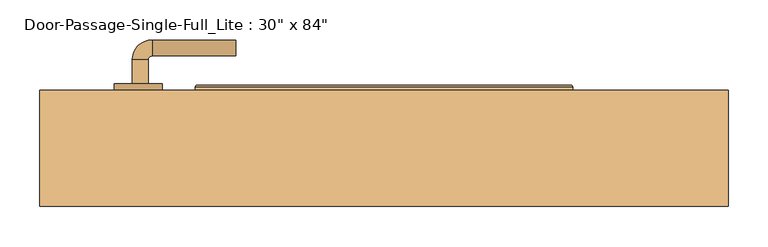
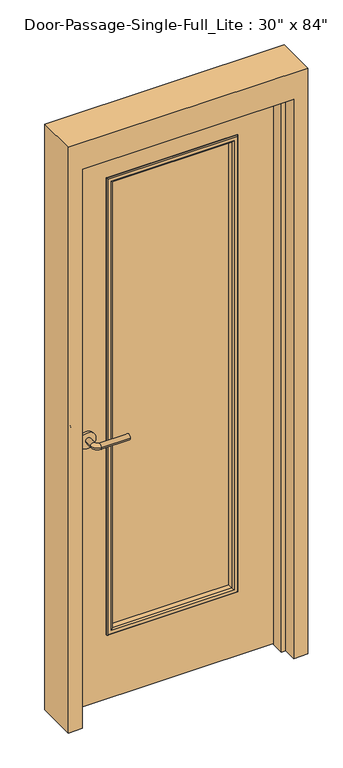
"""IFC4 building model written with IfcOpenShell, lengths in millimetres: door geometry."""

from ifc_helpers import new_model, si_unit, point, frame, frame_2d, origin, place, context, project, spatial, polyline, circle_curve, ellipse_curve, trimmed, segment, composite_curve, outline, extrude, faceted_brep, source, transform, mapped, element, save
from ifc_brep_helpers import plane_surface, cylinder_surface, revolved_surface, advanced_brep


def door_5761e9ac(model_context):
    return source(origin(), model_context, "Body", "SolidModel", [
        advanced_brep(
        [(-315.990625, 42.8, 1016.0), (-295.990625, 42.8, 1016.0), (-295.990625, 12.8, 1016.0), (-315.990625, 12.8, 1016.0), (-290.990625, 7.8, 1016.0), (-290.990625, -12.2, 1016.0), (-185.990625, -12.2, 1016.0), (-185.990625, 7.8, 1016.0)],
        [
            (0, 1, circle_curve(frame((-305.990625, 42.8, 1016.0), z_axis=(0.0, 1.0, 0.0), x_axis=(1.0, 0.0, 0.0)), 10.0)),
            (1, 0, circle_curve(frame((-305.990625, 42.8, 1016.0), z_axis=(0.0, 1.0, 0.0), x_axis=(1.0, 0.0, 0.0)), 10.0)),
            (1, 2),
            (2, 3, circle_curve(frame((-305.990625, 12.8, 1016.0), z_axis=(0.0, 1.0, 0.0), x_axis=(1.0, 0.0, 0.0)), 10.0)),
            (3, 0),
            (3, 2, circle_curve(frame((-305.990625, 12.8, 1016.0), z_axis=(0.0, 1.0, 0.0), x_axis=(1.0, 0.0, 0.0)), 10.0)),
            (4, 5, circle_curve(frame((-290.990625, -2.2, 1016.0), z_axis=(-1.0, 0.0, 0.0), x_axis=(0.0, 1.0, 0.0)), 10.0)),
            (5, 3, circle_curve(frame((-290.990625, 12.8, 1016.0), z_axis=(0.0, 0.0, -1.0), x_axis=(-1.0, 0.0, 0.0)), 25.0)),
            (2, 4, circle_curve(frame((-290.990625, 12.8, 1016.0), z_axis=(0.0, 0.0, 1.0), x_axis=(-1.0, 0.0, 0.0)), 5.0)),
            (5, 4, circle_curve(frame((-290.990625, -2.2, 1016.0), z_axis=(-1.0, 0.0, 0.0), x_axis=(0.0, 1.0, 0.0)), 10.0)),
            (6, 7, circle_curve(frame((-185.990625, -2.2, 1016.0), z_axis=(1.0, 0.0, 0.0), x_axis=(0.0, 1.0, 0.0)), 10.0)),
            (7, 6, circle_curve(frame((-185.990625, -2.2, 1016.0), z_axis=(1.0, 0.0, 0.0), x_axis=(0.0, 1.0, 0.0)), 10.0)),
            (4, 7),
            (6, 5),
        ],
        [
            plane_surface(frame((-305.990625, 42.8, 1016.0), z_axis=(0.0, 1.0, 0.0), x_axis=(0.0, 0.0, 1.0))),
            cylinder_surface(frame((-305.990625, 42.8, 1016.0), z_axis=(0.0, 1.0, 0.0), x_axis=(1.0, 0.0, 0.0)), 10.0),
            revolved_surface(trimmed(ellipse_curve(frame((-305.990625, 12.8, 1016.0), z_axis=(0.0, -1.0, 0.0), x_axis=(1.0, 0.0, 0.0)), 10.0, 10.0), [point((-315.990625, 12.8, 1016.0))], [point((-295.990625, 12.8, 1016.0))], True, "CARTESIAN"), (-290.990625, 12.8, 1016.0), (0.0, 0.0, -1.0)),
            revolved_surface(trimmed(ellipse_curve(frame((-305.990625, 12.8, 1016.0), z_axis=(0.0, -1.0, 0.0), x_axis=(1.0, 0.0, 0.0)), 10.0, 10.0), [point((-295.990625, 12.8, 1016.0))], [point((-315.990625, 12.8, 1016.0))], True, "CARTESIAN"), (-290.990625, 12.8, 1016.0), (0.0, 0.0, -1.0)),
            plane_surface(frame((-185.990625, -2.2, 1016.0), z_axis=(1.0, 0.0, 0.0), x_axis=(0.0, 0.0, 1.0))),
            cylinder_surface(frame((-290.990625, -2.2, 1016.0), z_axis=(-1.0, 0.0, 0.0), x_axis=(0.0, 1.0, 0.0)), 10.0),
        ],
        [
            (0, [[1, 2]]),
            (1, [[3, 4, 5, -2]]),
            (1, [[-5, 6, -3, -1]]),
            (2, [[7, 8, -4, 9]]),
            (3, [[10, -9, -6, -8]]),
            (4, [[11, 12]]),
            (5, [[13, -11, 14, -7]]),
            (5, [[-14, -12, -13, -10]]),
        ],
    ),
        extrude(outline(composite_curve([segment(trimmed(circle_curve(frame_2d((1016.0, -308.490625)), 30.0), [point((1016.0, -338.490625))], [point((1016.0, -278.490625))], False, "CARTESIAN"), True, "CONTINUOUS"), segment(trimmed(circle_curve(frame_2d((1016.0, -308.490625)), 30.0), [point((1016.0, -278.490625))], [point((1016.0, -338.490625))], False, "CARTESIAN"), True, "CONTINUOUS")], self_intersect=False)), frame((0.0, 42.8, 0.0), z_axis=(0.0, 1.0, 0.0), x_axis=(0.0, 0.0, 1.0)), (0.0, 0.0, 1.0), 8.0),
        advanced_brep(
        [(-315.990625, 103.25, 1016.0), (-295.990625, 103.25, 1016.0), (-315.990625, 133.25, 1016.0), (-295.990625, 133.25, 1016.0), (-290.990625, 138.25, 1016.0), (-290.990625, 158.25, 1016.0), (-185.990625, 158.25, 1016.0), (-185.990625, 138.25, 1016.0)],
        [
            (0, 1, circle_curve(frame((-305.990625, 103.25, 1016.0), z_axis=(0.0, -1.0, 0.0), x_axis=(1.0, 0.0, 0.0)), 10.0)),
            (1, 0, circle_curve(frame((-305.990625, 103.25, 1016.0), z_axis=(0.0, -1.0, 0.0), x_axis=(1.0, 0.0, 0.0)), 10.0)),
            (0, 2),
            (2, 3, circle_curve(frame((-305.990625, 133.25, 1016.0), z_axis=(0.0, -1.0, 0.0), x_axis=(1.0, 0.0, 0.0)), 10.0)),
            (3, 1),
            (3, 2, circle_curve(frame((-305.990625, 133.25, 1016.0), z_axis=(0.0, -1.0, 0.0), x_axis=(1.0, 0.0, 0.0)), 10.0)),
            (4, 3, circle_curve(frame((-290.990625, 133.25, 1016.0), z_axis=(0.0, 0.0, 1.0), x_axis=(-1.0, 0.0, 0.0)), 5.0)),
            (2, 5, circle_curve(frame((-290.990625, 133.25, 1016.0), z_axis=(0.0, 0.0, -1.0), x_axis=(-1.0, 0.0, 0.0)), 25.0)),
            (5, 4, circle_curve(frame((-290.990625, 148.25, 1016.0), z_axis=(-1.0, 0.0, 0.0), x_axis=(0.0, -1.0, 0.0)), 10.0)),
            (4, 5, circle_curve(frame((-290.990625, 148.25, 1016.0), z_axis=(-1.0, 0.0, 0.0), x_axis=(0.0, -1.0, 0.0)), 10.0)),
            (6, 7, circle_curve(frame((-185.990625, 148.25, 1016.0), z_axis=(1.0, 0.0, 0.0), x_axis=(0.0, -1.0, 0.0)), 10.0)),
            (7, 6, circle_curve(frame((-185.990625, 148.25, 1016.0), z_axis=(1.0, 0.0, 0.0), x_axis=(0.0, -1.0, 0.0)), 10.0)),
            (5, 6),
            (7, 4),
        ],
        [
            plane_surface(frame((-305.990625, 103.25, 1016.0), z_axis=(0.0, -1.0, 0.0), x_axis=(0.0, 0.0, 1.0))),
            cylinder_surface(frame((-305.990625, 103.25, 1016.0), z_axis=(0.0, -1.0, 0.0), x_axis=(1.0, 0.0, 0.0)), 10.0),
            revolved_surface(trimmed(ellipse_curve(frame((-305.990625, 133.25, 1016.0), z_axis=(0.0, -1.0, 0.0), x_axis=(1.0, 0.0, 0.0)), 10.0, 10.0), [point((-315.990625, 133.25, 1016.0))], [point((-295.990625, 133.25, 1016.0))], True, "CARTESIAN"), (-290.990625, 133.25, 1016.0), (0.0, 0.0, -1.0)),
            revolved_surface(trimmed(ellipse_curve(frame((-305.990625, 133.25, 1016.0), z_axis=(0.0, -1.0, 0.0), x_axis=(1.0, 0.0, 0.0)), 10.0, 10.0), [point((-295.990625, 133.25, 1016.0))], [point((-315.990625, 133.25, 1016.0))], True, "CARTESIAN"), (-290.990625, 133.25, 1016.0), (0.0, 0.0, -1.0)),
            plane_surface(frame((-185.990625, 148.25, 1016.0), z_axis=(1.0, 0.0, 0.0), x_axis=(0.0, 0.0, 1.0))),
            cylinder_surface(frame((-290.990625, 148.25, 1016.0), z_axis=(-1.0, 0.0, 0.0), x_axis=(0.0, -1.0, 0.0)), 10.0),
        ],
        [
            (0, [[1, 2]]),
            (1, [[-1, 3, 4, 5]]),
            (1, [[-2, -5, 6, -3]]),
            (2, [[7, -4, 8, 9]]),
            (3, [[-8, -6, -7, 10]]),
            (4, [[11, 12]]),
            (5, [[-9, 13, -12, 14]]),
            (5, [[-10, -14, -11, -13]]),
        ],
    ),
        extrude(outline(composite_curve([segment(trimmed(circle_curve(frame_2d((1016.0, -308.490625)), 30.0), [point((1016.0, -338.490625))], [point((1016.0, -278.490625))], False, "CARTESIAN"), True, "CONTINUOUS"), segment(trimmed(circle_curve(frame_2d((1016.0, -308.490625)), 30.0), [point((1016.0, -278.490625))], [point((1016.0, -338.490625))], False, "CARTESIAN"), True, "CONTINUOUS")], self_intersect=False)), frame((0.0, 95.25, 0.0), z_axis=(0.0, 1.0, 0.0), x_axis=(0.0, 0.0, 1.0)), (0.0, 0.0, 1.0), 8.0),
        extrude(outline(polyline([(2133.6, -381.0), (0.0, -381.0), (0.0, 381.0), (2133.6, 381.0), (2133.6, -381.0)]), holes=[polyline([(1981.2, -228.6), (1981.2, 228.6), (254.0, 228.6), (254.0, -228.6), (1981.2, -228.6)])]), frame((0.0, 50.8, 0.0), z_axis=(0.0, 1.0, 0.0), x_axis=(0.0, 0.0, 1.0)), (0.0, 0.0, 1.0), 44.45),
        faceted_brep([(381.0, 46.0375, 0.0), (381.0, 95.25, 0.0), (431.8, 95.25, 0.0), (431.8, -50.8, 0.0), (381.0, -50.8, 0.0), (381.0, -1.5875, 0.0), (365.125, -1.5875, 0.0), (365.125, 46.0375, 0.0), (381.0, 46.0375, 2133.6), (381.0, 95.25, 2133.6), (-381.0, 95.25, 2133.6), (-381.0, 95.25, 0.0), (-431.8, 95.25, 0.0), (-431.8, 95.25, 2235.2), (431.8, 95.25, 2235.2), (431.8, -50.8, 2235.2), (-431.8, -50.8, 2235.2), (-431.8, -50.8, 0.0), (-381.0, -50.8, 0.0), (-381.0, -50.8, 2133.6), (381.0, -50.8, 2133.6), (381.0, -1.5875, 2133.6), (-381.0, -1.5875, 2133.6), (-381.0, -1.5875, 0.0), (-365.125, -1.5875, 0.0), (-365.125, -1.5875, 2117.725), (365.125, -1.5875, 2117.725), (365.125, 46.0375, 2117.725), (-365.125, 46.0375, 2117.725), (-365.125, 46.0375, 0.0), (-381.0, 46.0375, 0.0), (-381.0, 46.0375, 2133.6)], [[[0, 1, 2, 3, 4, 5, 6, 7]], [[1, 0, 8, 9]], [[2, 1, 9, 10, 11, 12, 13, 14]], [[3, 2, 14, 15]], [[4, 3, 15, 16, 17, 18, 19, 20]], [[5, 4, 20, 21]], [[6, 5, 21, 22, 23, 24, 25, 26]], [[7, 6, 26, 27]], [[0, 7, 27, 28, 29, 30, 31, 8]], [[9, 8, 31, 10]], [[20, 19, 22, 21]], [[26, 25, 28, 27]], [[12, 11, 30, 29, 24, 23, 18, 17]], [[11, 10, 31, 30]], [[13, 12, 17, 16]], [[19, 18, 23, 22]], [[25, 24, 29, 28]], [[15, 14, 13, 16]]]),
        extrude(outline(polyline([(228.6, 69.85), (-228.6, 69.85), (-228.6, 76.2), (228.6, 76.2), (228.6, 69.85)])), frame((0.0, 0.0, 254.0), z_axis=(0.0, 0.0, 1.0), x_axis=(1.0, 0.0, 0.0)), (0.0, 0.0, 1.0), 1727.2),
        advanced_brep(
        [(-228.6, 76.2, 1981.2), (-228.6, 95.25, 1981.2), (-228.6, 95.25, 254.0), (-228.6, 76.2, 254.0), (-216.6, 96.25, 1969.2), (-216.6, 76.2, 1969.2), (-216.6, 76.2, 266.0), (-216.6, 96.25, 266.0), (-221.6, 101.25, 1974.2), (-221.6, 101.25, 261.0), (-236.6, 99.25, 1989.2), (-234.6, 101.25, 1987.2), (-234.6, 101.25, 248.0), (-236.6, 99.25, 246.0), (-236.6, 95.25, 1989.2), (-236.6, 95.25, 246.0), (228.6, 95.25, 254.0), (228.6, 76.2, 254.0), (216.6, 76.2, 266.0), (216.6, 96.25, 266.0), (221.6, 101.25, 261.0), (234.6, 101.25, 248.0), (236.6, 99.25, 246.0), (236.6, 95.25, 246.0), (228.6, 95.25, 1981.2), (228.6, 76.2, 1981.2), (216.6, 76.2, 1969.2), (216.6, 96.25, 1969.2), (221.6, 101.25, 1974.2), (234.6, 101.25, 1987.2), (236.6, 99.25, 1989.2), (236.6, 95.25, 1989.2)],
        [
            (0, 1),
            (1, 2),
            (2, 3),
            (3, 0),
            (4, 5),
            (5, 6),
            (6, 7),
            (7, 4),
            (8, 4, ellipse_curve(frame((-221.6, 96.25, 1974.2), z_axis=(-0.7071067811865475, 0.0, -0.7071067811865475), x_axis=(-0.7071067811865474, 0.0, 0.7071067811865476)), 7.0710678, 5.0)),
            (7, 9, ellipse_curve(frame((-221.6, 96.25, 261.0), z_axis=(-0.7071067811865475, 0.0, 0.7071067811865475), x_axis=(0.7071067811865474, 0.0, 0.7071067811865476)), 7.0710678, 5.0)),
            (9, 8),
            (10, 11, ellipse_curve(frame((-234.6, 99.25, 1987.2), z_axis=(-0.7071067811865475, 0.0, -0.7071067811865475), x_axis=(-0.7071067811865474, 0.0, 0.7071067811865476)), 2.8284271, 2.0)),
            (11, 12),
            (12, 13, ellipse_curve(frame((-234.6, 99.25, 248.0), z_axis=(-0.7071067811865475, 0.0, 0.7071067811865475), x_axis=(0.7071067811865474, 0.0, 0.7071067811865476)), 2.8284271, 2.0)),
            (13, 10),
            (14, 10),
            (13, 15),
            (15, 14),
            (2, 16),
            (16, 17),
            (17, 3),
            (6, 18),
            (18, 19),
            (19, 7),
            (19, 20, ellipse_curve(frame((221.6, 96.25, 261.0), z_axis=(-0.7071067811865475, 0.0, -0.7071067811865475), x_axis=(-0.7071067811865476, 0.0, 0.7071067811865474)), 7.0710678, 5.0)),
            (20, 9),
            (12, 21),
            (21, 22, ellipse_curve(frame((234.6, 99.25, 248.0), z_axis=(-0.7071067811865475, 0.0, -0.7071067811865475), x_axis=(-0.7071067811865476, 0.0, 0.7071067811865474)), 2.8284271, 2.0)),
            (22, 13),
            (22, 23),
            (23, 15),
            (16, 24),
            (24, 25),
            (25, 17),
            (18, 26),
            (26, 27),
            (27, 19),
            (27, 28, ellipse_curve(frame((221.6, 96.25, 1974.2), z_axis=(0.7071067811865475, 0.0, -0.7071067811865475), x_axis=(-0.7071067811865474, 0.0, -0.7071067811865476)), 7.0710678, 5.0)),
            (28, 20),
            (21, 29),
            (29, 30, ellipse_curve(frame((234.6, 99.25, 1987.2), z_axis=(0.7071067811865475, 0.0, -0.7071067811865475), x_axis=(-0.7071067811865474, 0.0, -0.7071067811865476)), 2.8284271, 2.0)),
            (30, 22),
            (30, 31),
            (31, 23),
            (31, 14),
            (1, 24),
            (0, 25),
            (5, 26),
            (4, 27),
            (8, 28),
            (11, 29),
            (10, 30),
        ],
        [
            plane_surface(frame((-228.6, 95.25, 1981.2), z_axis=(-1.0, 0.0, 0.0), x_axis=(0.0, 0.0, -1.0))),
            plane_surface(frame((-216.6, 76.2, 1969.2), z_axis=(1.0, 0.0, 0.0), x_axis=(0.0, 0.0, -1.0))),
            cylinder_surface(frame((-221.6, 96.25, 1981.2), z_axis=(0.0, 0.0, 1.0), x_axis=(-1.0, 0.0, 0.0)), 5.0),
            cylinder_surface(frame((-234.6, 99.25, 1981.2), z_axis=(0.0, 0.0, 1.0), x_axis=(-1.0, 0.0, 0.0)), 2.0),
            plane_surface(frame((-236.6, 99.25, 1989.2), z_axis=(-1.0, 0.0, 0.0), x_axis=(0.0, 0.0, -1.0))),
            plane_surface(frame((-228.6, 95.25, 254.0), z_axis=(0.0, 0.0, -1.0), x_axis=(1.0, 0.0, 0.0))),
            plane_surface(frame((-216.6, 76.2, 266.0), z_axis=(0.0, 0.0, 1.0), x_axis=(1.0, 0.0, 0.0))),
            cylinder_surface(frame((-228.6, 96.25, 261.0), z_axis=(-1.0, 0.0, 0.0), x_axis=(0.0, 0.0, -1.0)), 5.0),
            cylinder_surface(frame((-228.6, 99.25, 248.0), z_axis=(-1.0, 0.0, 0.0), x_axis=(0.0, 0.0, -1.0)), 2.0),
            plane_surface(frame((-236.6, 99.25, 246.0), z_axis=(0.0, 0.0, -1.0), x_axis=(1.0, 0.0, 0.0))),
            plane_surface(frame((228.6, 95.25, 254.0), z_axis=(1.0, 0.0, 0.0), x_axis=(0.0, 0.0, 1.0))),
            plane_surface(frame((216.6, 76.2, 266.0), z_axis=(-1.0, 0.0, 0.0), x_axis=(0.0, 0.0, 1.0))),
            cylinder_surface(frame((221.6, 96.25, 254.0), z_axis=(0.0, 0.0, -1.0), x_axis=(1.0, 0.0, 0.0)), 5.0),
            cylinder_surface(frame((234.6, 99.25, 254.0), z_axis=(0.0, 0.0, -1.0), x_axis=(1.0, 0.0, 0.0)), 2.0),
            plane_surface(frame((236.6, 99.25, 246.0), z_axis=(1.0, 0.0, 0.0), x_axis=(0.0, 0.0, 1.0))),
            plane_surface(frame((236.6, 95.25, 1989.2), z_axis=(0.0, -1.0, 0.0), x_axis=(-1.0, 0.0, 0.0))),
            plane_surface(frame((228.6, 95.25, 1981.2), z_axis=(0.0, 0.0, 1.0), x_axis=(-1.0, 0.0, 0.0))),
            plane_surface(frame((228.6, 76.2, 1981.2), z_axis=(0.0, -1.0, 0.0), x_axis=(-1.0, 0.0, 0.0))),
            plane_surface(frame((216.6, 76.2, 1969.2), z_axis=(0.0, 0.0, -1.0), x_axis=(-1.0, 0.0, 0.0))),
            cylinder_surface(frame((228.6, 96.25, 1974.2), z_axis=(1.0, 0.0, 0.0), x_axis=(0.0, 0.0, 1.0)), 5.0),
            plane_surface(frame((221.6, 101.25, 1974.2), z_axis=(0.0, 1.0, 0.0), x_axis=(-1.0, 0.0, 0.0))),
            cylinder_surface(frame((228.6, 99.25, 1987.2), z_axis=(1.0, 0.0, 0.0), x_axis=(0.0, 0.0, 1.0)), 2.0),
            plane_surface(frame((236.6, 99.25, 1989.2), z_axis=(0.0, 0.0, 1.0), x_axis=(-1.0, 0.0, 0.0))),
        ],
        [
            (0, [[1, 2, 3, 4]]),
            (1, [[5, 6, 7, 8]]),
            (2, [[9, -8, 10, 11]]),
            (3, [[12, 13, 14, 15]]),
            (4, [[16, -15, 17, 18]]),
            (5, [[-3, 19, 20, 21]]),
            (6, [[-7, 22, 23, 24]]),
            (7, [[-10, -24, 25, 26]]),
            (8, [[-14, 27, 28, 29]]),
            (9, [[-17, -29, 30, 31]]),
            (10, [[-20, 32, 33, 34]]),
            (11, [[-23, 35, 36, 37]]),
            (12, [[-25, -37, 38, 39]]),
            (13, [[-28, 40, 41, 42]]),
            (14, [[-30, -42, 43, 44]]),
            (15, [[-31, -44, 45, -18], [46, -32, -19, -2]]),
            (16, [[-33, -46, -1, 47]]),
            (17, [[-21, -34, -47, -4], [48, -35, -22, -6]]),
            (18, [[-36, -48, -5, 49]]),
            (19, [[-38, -49, -9, 50]]),
            (20, [[51, -40, -27, -13], [-26, -39, -50, -11]]),
            (21, [[-41, -51, -12, 52]]),
            (22, [[-43, -52, -16, -45]]),
        ],
    ),
        advanced_brep(
        [(-228.6, 69.85, 254.0), (-228.6, 50.8, 254.0), (-228.6, 50.8, 1981.2), (-228.6, 69.85, 1981.2), (-216.6, 49.8, 266.0), (-216.6, 69.85, 266.0), (-216.6, 69.85, 1969.2), (-216.6, 49.8, 1969.2), (-221.6, 44.8, 261.0), (-221.6, 44.8, 1974.2), (-236.6, 46.8, 246.0), (-234.6, 44.8, 248.0), (-234.6, 44.8, 1987.2), (-236.6, 46.8, 1989.2), (-236.6, 50.8, 246.0), (-236.6, 50.8, 1989.2), (228.6, 50.8, 1981.2), (228.6, 69.85, 1981.2), (216.6, 69.85, 1969.2), (216.6, 49.8, 1969.2), (221.6, 44.8, 1974.2), (234.6, 44.8, 1987.2), (236.6, 46.8, 1989.2), (236.6, 50.8, 1989.2), (228.6, 50.8, 254.0), (228.6, 69.85, 254.0), (216.6, 69.85, 266.0), (216.6, 49.8, 266.0), (221.6, 44.8, 261.0), (234.6, 44.8, 248.0), (236.6, 46.8, 246.0), (236.6, 50.8, 246.0)],
        [
            (0, 1),
            (1, 2),
            (2, 3),
            (3, 0),
            (4, 5),
            (5, 6),
            (6, 7),
            (7, 4),
            (8, 4, ellipse_curve(frame((-221.6, 49.8, 261.0), z_axis=(-0.7071067811865475, 0.0, 0.7071067811865475), x_axis=(-0.7071067811865474, 0.0, -0.7071067811865476)), 7.0710678, 5.0)),
            (7, 9, ellipse_curve(frame((-221.6, 49.8, 1974.2), z_axis=(-0.7071067811865475, 0.0, -0.7071067811865475), x_axis=(0.7071067811865474, 0.0, -0.7071067811865476)), 7.0710678, 5.0)),
            (9, 8),
            (10, 11, ellipse_curve(frame((-234.6, 46.8, 248.0), z_axis=(-0.7071067811865475, 0.0, 0.7071067811865475), x_axis=(-0.7071067811865474, 0.0, -0.7071067811865476)), 2.8284271, 2.0)),
            (11, 12),
            (12, 13, ellipse_curve(frame((-234.6, 46.8, 1987.2), z_axis=(-0.7071067811865475, 0.0, -0.7071067811865475), x_axis=(0.7071067811865474, 0.0, -0.7071067811865476)), 2.8284271, 2.0)),
            (13, 10),
            (14, 10),
            (13, 15),
            (15, 14),
            (2, 16),
            (16, 17),
            (17, 3),
            (6, 18),
            (18, 19),
            (19, 7),
            (19, 20, ellipse_curve(frame((221.6, 49.8, 1974.2), z_axis=(-0.7071067811865475, 0.0, 0.7071067811865475), x_axis=(-0.7071067811865476, 0.0, -0.7071067811865474)), 7.0710678, 5.0)),
            (20, 9),
            (12, 21),
            (21, 22, ellipse_curve(frame((234.6, 46.8, 1987.2), z_axis=(-0.7071067811865475, 0.0, 0.7071067811865475), x_axis=(-0.7071067811865476, 0.0, -0.7071067811865474)), 2.8284271, 2.0)),
            (22, 13),
            (22, 23),
            (23, 15),
            (16, 24),
            (24, 25),
            (25, 17),
            (18, 26),
            (26, 27),
            (27, 19),
            (27, 28, ellipse_curve(frame((221.6, 49.8, 261.0), z_axis=(0.7071067811865475, 0.0, 0.7071067811865475), x_axis=(-0.7071067811865474, 0.0, 0.7071067811865476)), 7.0710678, 5.0)),
            (28, 20),
            (21, 29),
            (29, 30, ellipse_curve(frame((234.6, 46.8, 248.0), z_axis=(0.7071067811865475, 0.0, 0.7071067811865475), x_axis=(-0.7071067811865474, 0.0, 0.7071067811865476)), 2.8284271, 2.0)),
            (30, 22),
            (30, 31),
            (31, 23),
            (31, 14),
            (1, 24),
            (0, 25),
            (5, 26),
            (4, 27),
            (8, 28),
            (11, 29),
            (10, 30),
        ],
        [
            plane_surface(frame((-228.6, 50.8, 254.0), z_axis=(-1.0, 0.0, 0.0), x_axis=(0.0, 0.0, 1.0))),
            plane_surface(frame((-216.6, 69.85, 266.0), z_axis=(1.0, 0.0, 0.0), x_axis=(0.0, 0.0, 1.0))),
            cylinder_surface(frame((-221.6, 49.8, 254.0), z_axis=(0.0, 0.0, -1.0), x_axis=(-1.0, 0.0, 0.0)), 5.0),
            cylinder_surface(frame((-234.6, 46.8, 254.0), z_axis=(0.0, 0.0, -1.0), x_axis=(-1.0, 0.0, 0.0)), 2.0),
            plane_surface(frame((-236.6, 46.8, 246.0), z_axis=(-1.0, 0.0, 0.0), x_axis=(0.0, 0.0, 1.0))),
            plane_surface(frame((-228.6, 50.8, 1981.2), z_axis=(0.0, 0.0, 1.0), x_axis=(1.0, 0.0, 0.0))),
            plane_surface(frame((-216.6, 69.85, 1969.2), z_axis=(0.0, 0.0, -1.0), x_axis=(1.0, 0.0, 0.0))),
            cylinder_surface(frame((-228.6, 49.8, 1974.2), z_axis=(-1.0, 0.0, 0.0), x_axis=(0.0, 0.0, 1.0)), 5.0),
            cylinder_surface(frame((-228.6, 46.8, 1987.2), z_axis=(-1.0, 0.0, 0.0), x_axis=(0.0, 0.0, 1.0)), 2.0),
            plane_surface(frame((-236.6, 46.8, 1989.2), z_axis=(0.0, 0.0, 1.0), x_axis=(1.0, 0.0, 0.0))),
            plane_surface(frame((228.6, 50.8, 1981.2), z_axis=(1.0, 0.0, 0.0), x_axis=(0.0, 0.0, -1.0))),
            plane_surface(frame((216.6, 69.85, 1969.2), z_axis=(-1.0, 0.0, 0.0), x_axis=(0.0, 0.0, -1.0))),
            cylinder_surface(frame((221.6, 49.8, 1981.2), z_axis=(0.0, 0.0, 1.0), x_axis=(1.0, 0.0, 0.0)), 5.0),
            cylinder_surface(frame((234.6, 46.8, 1981.2), z_axis=(0.0, 0.0, 1.0), x_axis=(1.0, 0.0, 0.0)), 2.0),
            plane_surface(frame((236.6, 46.8, 1989.2), z_axis=(1.0, 0.0, 0.0), x_axis=(0.0, 0.0, -1.0))),
            plane_surface(frame((236.6, 50.8, 246.0), z_axis=(0.0, 1.0, 0.0), x_axis=(-1.0, 0.0, 0.0))),
            plane_surface(frame((228.6, 50.8, 254.0), z_axis=(0.0, 0.0, -1.0), x_axis=(-1.0, 0.0, 0.0))),
            plane_surface(frame((228.6, 69.85, 254.0), z_axis=(0.0, 1.0, 0.0), x_axis=(-1.0, 0.0, 0.0))),
            plane_surface(frame((216.6, 69.85, 266.0), z_axis=(0.0, 0.0, 1.0), x_axis=(-1.0, 0.0, 0.0))),
            cylinder_surface(frame((228.6, 49.8, 261.0), z_axis=(1.0, 0.0, 0.0), x_axis=(0.0, 0.0, -1.0)), 5.0),
            plane_surface(frame((221.6, 44.8, 261.0), z_axis=(0.0, -1.0, 0.0), x_axis=(-1.0, 0.0, 0.0))),
            cylinder_surface(frame((228.6, 46.8, 248.0), z_axis=(1.0, 0.0, 0.0), x_axis=(0.0, 0.0, -1.0)), 2.0),
            plane_surface(frame((236.6, 46.8, 246.0), z_axis=(0.0, 0.0, -1.0), x_axis=(-1.0, 0.0, 0.0))),
        ],
        [
            (0, [[1, 2, 3, 4]]),
            (1, [[5, 6, 7, 8]]),
            (2, [[9, -8, 10, 11]]),
            (3, [[12, 13, 14, 15]]),
            (4, [[16, -15, 17, 18]]),
            (5, [[-3, 19, 20, 21]]),
            (6, [[-7, 22, 23, 24]]),
            (7, [[-10, -24, 25, 26]]),
            (8, [[-14, 27, 28, 29]]),
            (9, [[-17, -29, 30, 31]]),
            (10, [[-20, 32, 33, 34]]),
            (11, [[-23, 35, 36, 37]]),
            (12, [[-25, -37, 38, 39]]),
            (13, [[-28, 40, 41, 42]]),
            (14, [[-30, -42, 43, 44]]),
            (15, [[-31, -44, 45, -18], [46, -32, -19, -2]]),
            (16, [[-33, -46, -1, 47]]),
            (17, [[-21, -34, -47, -4], [48, -35, -22, -6]]),
            (18, [[-36, -48, -5, 49]]),
            (19, [[-38, -49, -9, 50]]),
            (20, [[51, -40, -27, -13], [-26, -39, -50, -11]]),
            (21, [[-41, -51, -12, 52]]),
            (22, [[-43, -52, -16, -45]]),
        ],
    ),
    ])


if __name__ == "__main__":
    model = new_model("IFC4")
    model_context = context("Model", 3, world=origin())
    ifc_project = project(units=[si_unit("LENGTHUNIT", "METRE", prefix="MILLI")], contexts=[model_context])
    site = spatial("IfcSite", under=ifc_project)
    building = spatial("IfcBuilding", under=site)
    placement = place(None, origin())
    door_shape = door_5761e9ac(model_context)
    element("IfcDoor", 1, ObjectType="Door-Passage-Single-Full_Lite : 30\" x 84\"", at=placement, inside=building, context=model_context, shape_type="MappedRepresentation", body=[
        mapped(door_shape, transform((0.0, 0.0, 0.0), x_axis=(1.0, 0.0, 0.0), y_axis=(0.0, 1.0, 0.0), z_axis=(0.0, 0.0, 1.0))),
    ])
    save(model, "model.ifc")

# Revit data of these elements
# Type "Door-Passage-Single-Full_Lite : 30\" x 84\""
#   Type Mark = "11"
#   Assembly Code = "B2030100"
#   Analytic Construction = "Wooden"
#   Thickness = 0' - 1 3/4"
#   Thermal Resistance (R) = 2.5876 (h·ft²·°F)/BTU
#   Swing Angle [instance default] = 90.00°
#   Strike Height = 3' - 4"
#   Rough Width [instance default] = 2' - 10"
#   Rough Height [instance default] = 7' - 4"
#   MF Opening Height [instance default] = 0' - 4"
#   MF Opening Width [instance default] = 0' - 4"
#   Inset Calculate [instance default] = 0' - 4"
#   Masonry Inset [instance default] = 0' - 1"
#   Height = 7' - 0"
#   Width = 2' - 6"
#   Heat Transfer Coefficient (U) = 0.3865 BTU/(h·ft²·°F)
#   Masonry Frame Depth = 0' - 5 3/4"
#   Masonry Frame [instance default] = yes
#   Function = 1
#   Dry Wall Frame [instance default] = no
#   Panel Material = Wood - Birch
#   Glazing = Glass
#   Glass Stop Material = Metal - Paint Finish - Grey
#   Frame Material = Metal - Paint Finish - Grey
#   Door Handle Material = Aluminum
#   Visual Light Transmittance = 0
#   Solar Heat Gain Coefficient = 0
#   Wall Closure = (empty or 0)
# Element 1 (IfcDoor, "Door-Passage-Single-Full_Lite : 30\" x 84\"")
#   Materials on its faces: "Metal - Paint Finish - Grey", "Aluminum", "Wood - Birch", "Glass"
# Materials
#   "Wood - Birch": class "Wood", colour RGB 166 116 52, transparency 0, Cost = 0
#   "Glass": class "Glass", colour RGB 0 128 192, transparency 0.75, Description = "Soda Lime Glass", Cost = 0
#   "Metal - Paint Finish - Grey": class "Paint", colour RGB 104 104 104, transparency 0, Cost = 0
#   "Aluminum": class "Metal", colour RGB 247 247 247, transparency 0, Description = "Aluminum 6061", Cost = 0
